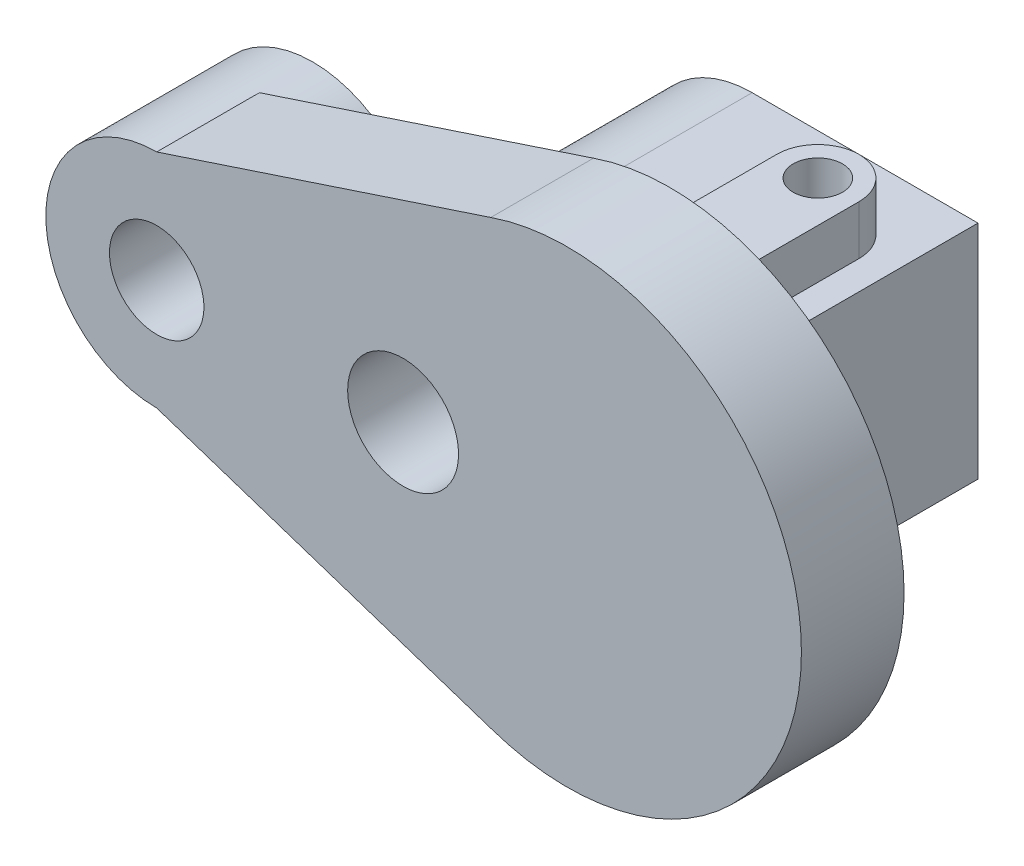
ISO-10303-21;
HEADER;
FILE_DESCRIPTION(('STEP AP214'),'2;1');
FILE_NAME('part.step','',(''),(''),'','','');
FILE_SCHEMA(('AUTOMOTIVE_DESIGN { 1 0 10303 214 1 1 1 1 }'));
ENDSEC;
DATA;
#1=APPLICATION_CONTEXT('core data for automotive mechanical design processes');
#2=APPLICATION_PROTOCOL_DEFINITION('international standard','automotive_design',2000,#1);
#3=PRODUCT_CONTEXT('',#1,'mechanical');
#4=PRODUCT('Part','Part','',(#3));
#5=PRODUCT_RELATED_PRODUCT_CATEGORY('part','',(#4));
#6=PRODUCT_DEFINITION_FORMATION('','',#4);
#7=PRODUCT_DEFINITION_CONTEXT('part definition',#1,'design');
#8=PRODUCT_DEFINITION('design','',#6,#7);
#9=PRODUCT_DEFINITION_SHAPE('','',#8);
#10=(LENGTH_UNIT() NAMED_UNIT(*) SI_UNIT(.MILLI.,.METRE.));
#11=(NAMED_UNIT(*) PLANE_ANGLE_UNIT() SI_UNIT($,.RADIAN.));
#12=(NAMED_UNIT(*) SI_UNIT($,.STERADIAN.) SOLID_ANGLE_UNIT());
#13=UNCERTAINTY_MEASURE_WITH_UNIT(LENGTH_MEASURE(1.E-05),#10,'distance_accuracy_value','');
#14=(GEOMETRIC_REPRESENTATION_CONTEXT(3) GLOBAL_UNCERTAINTY_ASSIGNED_CONTEXT((#13)) GLOBAL_UNIT_ASSIGNED_CONTEXT((#10,
#11,#12)) REPRESENTATION_CONTEXT('',''));
#15=CARTESIAN_POINT('',(0.,0.,0.));
#16=DIRECTION('',(0.,0.,1.));
#17=DIRECTION('',(1.,0.,0.));
#18=AXIS2_PLACEMENT_3D('',#15,#16,#17);
#19=CARTESIAN_POINT('',(115000.,27000.,-66000.));
#20=DIRECTION('',(0.,-1.,0.));
#21=DIRECTION('',(0.,0.,-1.));
#22=AXIS2_PLACEMENT_3D('',#19,#20,#21);
#23=PLANE('',#22);
#24=DIRECTION('',(0.,0.,-1.));
#25=VECTOR('',#24,1.);
#26=CARTESIAN_POINT('',(108000.,27000.,-6000.));
#27=LINE('',#26,#25);
#28=CARTESIAN_POINT('',(108000.,27000.,-11000.));
#29=VERTEX_POINT('',#28);
#30=CARTESIAN_POINT('',(108000.,27000.,-44000.));
#31=VERTEX_POINT('',#30);
#32=EDGE_CURVE('E187',#29,#31,#27,.T.);
#33=ORIENTED_EDGE('',*,*,#32,.F.);
#34=DIRECTION('',(1.,0.,0.));
#35=VECTOR('',#34,1.);
#36=CARTESIAN_POINT('',(-27000.001,27000.,-11000.));
#37=LINE('',#36,#35);
#38=CARTESIAN_POINT('',(115000.,27000.,-11000.));
#39=VERTEX_POINT('',#38);
#40=EDGE_CURVE('E204',#29,#39,#37,.T.);
#41=ORIENTED_EDGE('',*,*,#40,.T.);
#42=DIRECTION('',(0.,0.,1.));
#43=VECTOR('',#42,1.);
#44=CARTESIAN_POINT('',(115000.,27000.,-66000.));
#45=LINE('',#44,#43);
#46=CARTESIAN_POINT('',(115000.,27000.,-66000.));
#47=VERTEX_POINT('',#46);
#48=EDGE_CURVE('E227',#47,#39,#45,.T.);
#49=ORIENTED_EDGE('',*,*,#48,.F.);
#50=DIRECTION('',(1.,0.,0.));
#51=VECTOR('',#50,1.);
#52=CARTESIAN_POINT('',(115000.,27000.,-66000.));
#53=LINE('',#52,#51);
#54=CARTESIAN_POINT('',(60000.,27000.,-66000.));
#55=VERTEX_POINT('',#54);
#56=EDGE_CURVE('E213',#55,#47,#53,.T.);
#57=ORIENTED_EDGE('',*,*,#56,.F.);
#58=DIRECTION('',(0.,0.,1.));
#59=VECTOR('',#58,1.);
#60=CARTESIAN_POINT('',(60000.,27000.,-66000.));
#61=LINE('',#60,#59);
#62=CARTESIAN_POINT('',(60000.,27000.,-11000.));
#63=VERTEX_POINT('',#62);
#64=EDGE_CURVE('E229',#55,#63,#61,.T.);
#65=ORIENTED_EDGE('',*,*,#64,.T.);
#66=CARTESIAN_POINT('',(88000.,27000.,-11000.));
#67=VERTEX_POINT('',#66);
#68=EDGE_CURVE('E201',#63,#67,#37,.T.);
#69=ORIENTED_EDGE('',*,*,#68,.T.);
#70=DIRECTION('',(0.,0.,1.));
#71=VECTOR('',#70,1.);
#72=CARTESIAN_POINT('',(88000.,27000.,-6000.));
#73=LINE('',#72,#71);
#74=CARTESIAN_POINT('',(88000.,27000.,-44000.));
#75=VERTEX_POINT('',#74);
#76=EDGE_CURVE('E563',#75,#67,#73,.T.);
#77=ORIENTED_EDGE('',*,*,#76,.F.);
#78=CARTESIAN_POINT('',(98000.,27000.,-44000.));
#79=DIRECTION('',(0.,1.,0.));
#80=DIRECTION('',(0.,0.,1.));
#81=AXIS2_PLACEMENT_3D('',#78,#79,#80);
#82=CIRCLE('',#81,10000.);
#83=EDGE_CURVE('E557',#31,#75,#82,.T.);
#84=ORIENTED_EDGE('',*,*,#83,.F.);
#85=EDGE_LOOP('',(#33,#41,#49,#57,#65,#69,#77,#84));
#86=FACE_BOUND('',#85,.T.);
#87=ADVANCED_FACE('F41',(#86),#23,.F.);
#88=CARTESIAN_POINT('',(98000.,-27000.,-44000.));
#89=DIRECTION('',(0.,-1.,0.));
#90=DIRECTION('',(0.,0.,-1.));
#91=AXIS2_PLACEMENT_3D('',#88,#89,#90);
#92=PLANE('',#91);
#93=DIRECTION('',(1.,0.,0.));
#94=VECTOR('',#93,1.);
#95=CARTESIAN_POINT('',(98000.,-27000.,-11000.));
#96=LINE('',#95,#94);
#97=CARTESIAN_POINT('',(88000.,-27000.,-11000.));
#98=VERTEX_POINT('',#97);
#99=CARTESIAN_POINT('',(108000.,-27000.,-11000.));
#100=VERTEX_POINT('',#99);
#101=EDGE_CURVE('E11',#98,#100,#96,.T.);
#102=ORIENTED_EDGE('',*,*,#101,.F.);
#103=DIRECTION('',(0.,0.,-1.));
#104=VECTOR('',#103,1.);
#105=CARTESIAN_POINT('',(88000.,-27000.,-6000.));
#106=LINE('',#105,#104);
#107=CARTESIAN_POINT('',(88000.,-27000.,-6000.));
#108=VERTEX_POINT('',#107);
#109=EDGE_CURVE('E252',#108,#98,#106,.T.);
#110=ORIENTED_EDGE('',*,*,#109,.F.);
#111=DIRECTION('',(-1.,0.,0.));
#112=VECTOR('',#111,1.);
#113=CARTESIAN_POINT('',(108000.,-27000.,-6000.));
#114=LINE('',#113,#112);
#115=CARTESIAN_POINT('',(108000.,-27000.,-6000.));
#116=VERTEX_POINT('',#115);
#117=EDGE_CURVE('E247',#116,#108,#114,.T.);
#118=ORIENTED_EDGE('',*,*,#117,.F.);
#119=DIRECTION('',(0.,0.,1.));
#120=VECTOR('',#119,1.);
#121=CARTESIAN_POINT('',(108000.,-27000.,-6000.));
#122=LINE('',#121,#120);
#123=EDGE_CURVE('E231',#100,#116,#122,.T.);
#124=ORIENTED_EDGE('',*,*,#123,.F.);
#125=EDGE_LOOP('',(#102,#110,#118,#124));
#126=FACE_BOUND('',#125,.T.);
#127=ADVANCED_FACE('F354',(#126),#92,.F.);
#128=CARTESIAN_POINT('',(0.,0.,-6000.));
#129=DIRECTION('',(0.,0.,1.));
#130=DIRECTION('',(1.,0.,0.));
#131=AXIS2_PLACEMENT_3D('',#128,#129,#130);
#132=PLANE('',#131);
#133=DIRECTION('',(0.,-1.,0.));
#134=VECTOR('',#133,1.);
#135=CARTESIAN_POINT('',(108000.,39000.,-6000.));
#136=LINE('',#135,#134);
#137=CARTESIAN_POINT('',(108000.,39000.,-6000.));
#138=VERTEX_POINT('',#137);
#139=CARTESIAN_POINT('',(108000.,27000.,-6000.));
#140=VERTEX_POINT('',#139);
#141=EDGE_CURVE('E57',#138,#140,#136,.T.);
#142=ORIENTED_EDGE('',*,*,#141,.F.);
#143=DIRECTION('',(1.,0.,0.));
#144=VECTOR('',#143,1.);
#145=CARTESIAN_POINT('',(108000.,39000.,-6000.));
#146=LINE('',#145,#144);
#147=CARTESIAN_POINT('',(88000.,39000.,-6000.));
#148=VERTEX_POINT('',#147);
#149=EDGE_CURVE('E58',#148,#138,#146,.T.);
#150=ORIENTED_EDGE('',*,*,#149,.F.);
#151=DIRECTION('',(0.,-1.,0.));
#152=VECTOR('',#151,1.);
#153=CARTESIAN_POINT('',(88000.,39000.,-6000.));
#154=LINE('',#153,#152);
#155=CARTESIAN_POINT('',(88000.,27000.,-6000.));
#156=VERTEX_POINT('',#155);
#157=EDGE_CURVE('E195',#148,#156,#154,.T.);
#158=ORIENTED_EDGE('',*,*,#157,.T.);
#159=DIRECTION('',(1.,0.,0.));
#160=VECTOR('',#159,1.);
#161=CARTESIAN_POINT('',(108000.,27000.,-6000.));
#162=LINE('',#161,#160);
#163=EDGE_CURVE('E179',#156,#140,#162,.T.);
#164=ORIENTED_EDGE('',*,*,#163,.T.);
#165=EDGE_LOOP('',(#142,#150,#158,#164));
#166=FACE_BOUND('',#165,.T.);
#167=DIRECTION('',(0.,1.,0.));
#168=VECTOR('',#167,1.);
#169=CARTESIAN_POINT('',(88000.,-39000.,-6000.));
#170=LINE('',#169,#168);
#171=CARTESIAN_POINT('',(88000.,-39000.,-6000.));
#172=VERTEX_POINT('',#171);
#173=EDGE_CURVE('E258',#172,#108,#170,.T.);
#174=ORIENTED_EDGE('',*,*,#173,.F.);
#175=DIRECTION('',(-1.,0.,0.));
#176=VECTOR('',#175,1.);
#177=CARTESIAN_POINT('',(108000.,-39000.,-6000.));
#178=LINE('',#177,#176);
#179=CARTESIAN_POINT('',(108000.,-39000.,-6000.));
#180=VERTEX_POINT('',#179);
#181=EDGE_CURVE('E240',#180,#172,#178,.T.);
#182=ORIENTED_EDGE('',*,*,#181,.F.);
#183=DIRECTION('',(0.,1.,0.));
#184=VECTOR('',#183,1.);
#185=CARTESIAN_POINT('',(108000.,-39000.,-6000.));
#186=LINE('',#185,#184);
#187=EDGE_CURVE('E261',#180,#116,#186,.T.);
#188=ORIENTED_EDGE('',*,*,#187,.T.);
#189=ORIENTED_EDGE('',*,*,#117,.T.);
#190=EDGE_LOOP('',(#174,#182,#188,#189));
#191=FACE_BOUND('',#190,.T.);
#192=CARTESIAN_POINT('',(0.,0.,-6000.));
#193=DIRECTION('',(0.,0.,-1.));
#194=DIRECTION('',(1.,0.,0.));
#195=AXIS2_PLACEMENT_3D('',#192,#193,#194);
#196=CIRCLE('',#195,27000.);
#197=CARTESIAN_POINT('',(0.,27000.,-6000.));
#198=VERTEX_POINT('',#197);
#199=CARTESIAN_POINT('',(0.,-27000.,-6000.));
#200=VERTEX_POINT('',#199);
#201=EDGE_CURVE('E267',#198,#200,#196,.T.);
#202=ORIENTED_EDGE('',*,*,#201,.F.);
#203=DIRECTION('',(-0.949568733780847,-0.313558957495777,0.));
#204=VECTOR('',#203,1.);
#205=CARTESIAN_POINT('',(0.,27000.,-6000.));
#206=LINE('',#205,#204);
#207=CARTESIAN_POINT('',(81360.2667835362,53866.1335684961,-6000.));
#208=VERTEX_POINT('',#207);
#209=EDGE_CURVE('E289',#208,#198,#206,.T.);
#210=ORIENTED_EDGE('',*,*,#209,.F.);
#211=CARTESIAN_POINT('',(100000.,0.,-6000.));
#212=DIRECTION('',(0.,0.,1.));
#213=DIRECTION('',(1.,0.,0.));
#214=AXIS2_PLACEMENT_3D('',#211,#212,#213);
#215=CIRCLE('',#214,57000.);
#216=CARTESIAN_POINT('',(81360.2667835362,-53866.1335684961,-6000.));
#217=VERTEX_POINT('',#216);
#218=EDGE_CURVE('E284',#217,#208,#215,.T.);
#219=ORIENTED_EDGE('',*,*,#218,.F.);
#220=DIRECTION('',(0.949568733780847,-0.313558957495777,0.));
#221=VECTOR('',#220,1.);
#222=CARTESIAN_POINT('',(0.,-27000.,-6000.));
#223=LINE('',#222,#221);
#224=EDGE_CURVE('E285',#200,#217,#223,.T.);
#225=ORIENTED_EDGE('',*,*,#224,.F.);
#226=EDGE_LOOP('',(#202,#210,#219,#225));
#227=FACE_BOUND('',#226,.T.);
#228=CARTESIAN_POINT('',(60000.,-1.4210854715202E-11,-6000.));
#229=DIRECTION('',(0.,0.,1.));
#230=DIRECTION('',(1.,0.,0.));
#231=AXIS2_PLACEMENT_3D('',#228,#229,#230);
#232=CIRCLE('',#231,13500.);
#233=CARTESIAN_POINT('',(73500.,-1.4210854715202E-11,-6000.));
#234=VERTEX_POINT('',#233);
#235=EDGE_CURVE('E47',#234,#234,#232,.T.);
#236=ORIENTED_EDGE('',*,*,#235,.T.);
#237=EDGE_LOOP('',(#236));
#238=FACE_BOUND('',#237,.T.);
#239=ADVANCED_FACE('F312',(#166,#191,#227,#238),#132,.F.);
#240=CARTESIAN_POINT('',(0.,0.,19000.));
#241=DIRECTION('',(0.,0.,-1.));
#242=DIRECTION('',(-1.,0.,0.));
#243=AXIS2_PLACEMENT_3D('',#240,#241,#242);
#244=CYLINDRICAL_SURFACE('',#243,27000.);
#245=CARTESIAN_POINT('',(0.,0.,19000.));
#246=DIRECTION('',(0.,0.,1.));
#247=DIRECTION('',(1.,0.,0.));
#248=AXIS2_PLACEMENT_3D('',#245,#246,#247);
#249=CIRCLE('',#248,27000.);
#250=CARTESIAN_POINT('',(0.,27000.,19000.));
#251=VERTEX_POINT('',#250);
#252=CARTESIAN_POINT('',(0.,-27000.,19000.));
#253=VERTEX_POINT('',#252);
#254=EDGE_CURVE('E275',#251,#253,#249,.T.);
#255=ORIENTED_EDGE('',*,*,#254,.F.);
#256=DIRECTION('',(0.,0.,1.));
#257=VECTOR('',#256,1.);
#258=CARTESIAN_POINT('',(0.,27000.,-6000.));
#259=LINE('',#258,#257);
#260=EDGE_CURVE('E287',#198,#251,#259,.T.);
#261=ORIENTED_EDGE('',*,*,#260,.F.);
#262=ORIENTED_EDGE('',*,*,#201,.T.);
#263=DIRECTION('',(0.,0.,1.));
#264=VECTOR('',#263,1.);
#265=CARTESIAN_POINT('',(0.,-27000.,-6000.));
#266=LINE('',#265,#264);
#267=EDGE_CURVE('E272',#200,#253,#266,.T.);
#268=ORIENTED_EDGE('',*,*,#267,.T.);
#269=EDGE_LOOP('',(#255,#261,#262,#268));
#270=FACE_BOUND('',#269,.T.);
#271=CARTESIAN_POINT('',(0.,0.,-19000.));
#272=DIRECTION('',(0.,0.,1.));
#273=DIRECTION('',(1.,0.,0.));
#274=AXIS2_PLACEMENT_3D('',#271,#272,#273);
#275=CIRCLE('',#274,27000.);
#276=CARTESIAN_POINT('',(27000.,0.,-19000.));
#277=VERTEX_POINT('',#276);
#278=EDGE_CURVE('E270',#277,#277,#275,.T.);
#279=ORIENTED_EDGE('',*,*,#278,.T.);
#280=EDGE_LOOP('',(#279));
#281=FACE_BOUND('',#280,.T.);
#282=ADVANCED_FACE('F323',(#270,#281),#244,.T.);
#283=CARTESIAN_POINT('',(0.,0.,19000.));
#284=DIRECTION('',(0.,0.,1.));
#285=DIRECTION('',(1.,0.,0.));
#286=AXIS2_PLACEMENT_3D('',#283,#284,#285);
#287=PLANE('',#286);
#288=CARTESIAN_POINT('',(0.,0.,19000.));
#289=DIRECTION('',(0.,0.,-1.));
#290=DIRECTION('',(-1.,0.,0.));
#291=AXIS2_PLACEMENT_3D('',#288,#289,#290);
#292=CIRCLE('',#291,11500.);
#293=CARTESIAN_POINT('',(-11500.,0.,19000.));
#294=VERTEX_POINT('',#293);
#295=EDGE_CURVE('E266',#294,#294,#292,.T.);
#296=ORIENTED_EDGE('',*,*,#295,.T.);
#297=EDGE_LOOP('',(#296));
#298=FACE_BOUND('',#297,.T.);
#299=CARTESIAN_POINT('',(60000.,-1.4210854715202E-11,19000.));
#300=DIRECTION('',(0.,0.,-1.));
#301=DIRECTION('',(-1.,0.,0.));
#302=AXIS2_PLACEMENT_3D('',#299,#300,#301);
#303=CIRCLE('',#302,13500.);
#304=CARTESIAN_POINT('',(46500.,-1.4210854715202E-11,19000.));
#305=VERTEX_POINT('',#304);
#306=EDGE_CURVE('E277',#305,#305,#303,.T.);
#307=ORIENTED_EDGE('',*,*,#306,.T.);
#308=EDGE_LOOP('',(#307));
#309=FACE_BOUND('',#308,.T.);
#310=ORIENTED_EDGE('',*,*,#254,.T.);
#311=DIRECTION('',(0.949568733780847,-0.313558957495777,0.));
#312=VECTOR('',#311,1.);
#313=CARTESIAN_POINT('',(0.,-27000.,19000.));
#314=LINE('',#313,#312);
#315=CARTESIAN_POINT('',(81360.2667835362,-53866.1335684961,19000.));
#316=VERTEX_POINT('',#315);
#317=EDGE_CURVE('E273',#253,#316,#314,.T.);
#318=ORIENTED_EDGE('',*,*,#317,.T.);
#319=CARTESIAN_POINT('',(100000.,0.,19000.));
#320=DIRECTION('',(0.,0.,1.));
#321=DIRECTION('',(1.,0.,0.));
#322=AXIS2_PLACEMENT_3D('',#319,#320,#321);
#323=CIRCLE('',#322,57000.);
#324=CARTESIAN_POINT('',(81360.2667835362,53866.1335684961,19000.));
#325=VERTEX_POINT('',#324);
#326=EDGE_CURVE('E292',#316,#325,#323,.T.);
#327=ORIENTED_EDGE('',*,*,#326,.T.);
#328=DIRECTION('',(-0.949568733780847,-0.313558957495777,0.));
#329=VECTOR('',#328,1.);
#330=CARTESIAN_POINT('',(0.,27000.,19000.));
#331=LINE('',#330,#329);
#332=EDGE_CURVE('E286',#325,#251,#331,.T.);
#333=ORIENTED_EDGE('',*,*,#332,.T.);
#334=EDGE_LOOP('',(#310,#318,#327,#333));
#335=FACE_BOUND('',#334,.T.);
#336=ADVANCED_FACE('F322',(#298,#309,#335),#287,.T.);
#337=CARTESIAN_POINT('',(0.,0.,-19000.));
#338=DIRECTION('',(0.,0.,1.));
#339=DIRECTION('',(1.,0.,0.));
#340=AXIS2_PLACEMENT_3D('',#337,#338,#339);
#341=PLANE('',#340);
#342=CARTESIAN_POINT('',(0.,0.,-19000.));
#343=DIRECTION('',(0.,0.,-1.));
#344=DIRECTION('',(-1.,0.,0.));
#345=AXIS2_PLACEMENT_3D('',#342,#343,#344);
#346=CIRCLE('',#345,11500.);
#347=CARTESIAN_POINT('',(-11500.,0.,-19000.));
#348=VERTEX_POINT('',#347);
#349=EDGE_CURVE('E283',#348,#348,#346,.T.);
#350=ORIENTED_EDGE('',*,*,#349,.F.);
#351=EDGE_LOOP('',(#350));
#352=FACE_BOUND('',#351,.T.);
#353=ORIENTED_EDGE('',*,*,#278,.F.);
#354=EDGE_LOOP('',(#353));
#355=FACE_BOUND('',#354,.T.);
#356=ADVANCED_FACE('F321',(#352,#355),#341,.F.);
#357=CARTESIAN_POINT('',(0.,27000.,-6000.));
#358=DIRECTION('',(-0.313558957495777,0.949568733780847,0.));
#359=DIRECTION('',(-0.949568733780847,-0.313558957495777,0.));
#360=AXIS2_PLACEMENT_3D('',#357,#358,#359);
#361=PLANE('',#360);
#362=ORIENTED_EDGE('',*,*,#332,.F.);
#363=DIRECTION('',(0.,0.,1.));
#364=VECTOR('',#363,1.);
#365=CARTESIAN_POINT('',(81360.2667835362,53866.1335684961,-6000.));
#366=LINE('',#365,#364);
#367=EDGE_CURVE('E281',#208,#325,#366,.T.);
#368=ORIENTED_EDGE('',*,*,#367,.F.);
#369=ORIENTED_EDGE('',*,*,#209,.T.);
#370=ORIENTED_EDGE('',*,*,#260,.T.);
#371=EDGE_LOOP('',(#362,#368,#369,#370));
#372=FACE_BOUND('',#371,.T.);
#373=ADVANCED_FACE('F345',(#372),#361,.T.);
#374=CARTESIAN_POINT('',(100000.,0.,-6000.));
#375=DIRECTION('',(0.,0.,1.));
#376=DIRECTION('',(1.,0.,0.));
#377=AXIS2_PLACEMENT_3D('',#374,#375,#376);
#378=CYLINDRICAL_SURFACE('',#377,57000.);
#379=ORIENTED_EDGE('',*,*,#326,.F.);
#380=DIRECTION('',(0.,0.,1.));
#381=VECTOR('',#380,1.);
#382=CARTESIAN_POINT('',(81360.2667835362,-53866.1335684961,-6000.));
#383=LINE('',#382,#381);
#384=EDGE_CURVE('E276',#217,#316,#383,.T.);
#385=ORIENTED_EDGE('',*,*,#384,.F.);
#386=ORIENTED_EDGE('',*,*,#218,.T.);
#387=ORIENTED_EDGE('',*,*,#367,.T.);
#388=EDGE_LOOP('',(#379,#385,#386,#387));
#389=FACE_BOUND('',#388,.T.);
#390=ADVANCED_FACE('F338',(#389),#378,.T.);
#391=CARTESIAN_POINT('',(0.,-27000.,-6000.));
#392=DIRECTION('',(-0.313558957495777,-0.949568733780847,0.));
#393=DIRECTION('',(0.949568733780847,-0.313558957495777,0.));
#394=AXIS2_PLACEMENT_3D('',#391,#392,#393);
#395=PLANE('',#394);
#396=ORIENTED_EDGE('',*,*,#317,.F.);
#397=ORIENTED_EDGE('',*,*,#267,.F.);
#398=ORIENTED_EDGE('',*,*,#224,.T.);
#399=ORIENTED_EDGE('',*,*,#384,.T.);
#400=EDGE_LOOP('',(#396,#397,#398,#399));
#401=FACE_BOUND('',#400,.T.);
#402=ADVANCED_FACE('F319',(#401),#395,.T.);
#403=CARTESIAN_POINT('',(60000.,-1.4210854715202E-11,19000.));
#404=DIRECTION('',(0.,0.,-1.));
#405=DIRECTION('',(-1.,0.,0.));
#406=AXIS2_PLACEMENT_3D('',#403,#404,#405);
#407=CYLINDRICAL_SURFACE('',#406,13500.);
#408=ORIENTED_EDGE('',*,*,#235,.F.);
#409=EDGE_LOOP('',(#408));
#410=FACE_BOUND('',#409,.T.);
#411=ORIENTED_EDGE('',*,*,#306,.F.);
#412=EDGE_LOOP('',(#411));
#413=FACE_BOUND('',#412,.T.);
#414=ADVANCED_FACE('F43',(#410,#413),#407,.F.);
#415=CARTESIAN_POINT('',(0.,0.,19000.));
#416=DIRECTION('',(0.,0.,-1.));
#417=DIRECTION('',(-1.,0.,0.));
#418=AXIS2_PLACEMENT_3D('',#415,#416,#417);
#419=CYLINDRICAL_SURFACE('',#418,11500.);
#420=ORIENTED_EDGE('',*,*,#295,.F.);
#421=EDGE_LOOP('',(#420));
#422=FACE_BOUND('',#421,.T.);
#423=ORIENTED_EDGE('',*,*,#349,.T.);
#424=EDGE_LOOP('',(#423));
#425=FACE_BOUND('',#424,.T.);
#426=ADVANCED_FACE('F320',(#422,#425),#419,.F.);
#427=CARTESIAN_POINT('',(108000.,-39000.,-6000.));
#428=DIRECTION('',(-1.,0.,0.));
#429=DIRECTION('',(0.,0.,1.));
#430=AXIS2_PLACEMENT_3D('',#427,#428,#429);
#431=PLANE('',#430);
#432=CARTESIAN_POINT('',(108000.,-27000.,-44000.));
#433=VERTEX_POINT('',#432);
#434=EDGE_CURVE('E246',#433,#100,#122,.T.);
#435=ORIENTED_EDGE('',*,*,#434,.T.);
#436=ORIENTED_EDGE('',*,*,#123,.T.);
#437=ORIENTED_EDGE('',*,*,#187,.F.);
#438=DIRECTION('',(0.,0.,1.));
#439=VECTOR('',#438,1.);
#440=CARTESIAN_POINT('',(108000.,-39000.,-6000.));
#441=LINE('',#440,#439);
#442=CARTESIAN_POINT('',(108000.,-39000.,-44000.));
#443=VERTEX_POINT('',#442);
#444=EDGE_CURVE('E234',#443,#180,#441,.T.);
#445=ORIENTED_EDGE('',*,*,#444,.F.);
#446=DIRECTION('',(0.,1.,0.));
#447=VECTOR('',#446,1.);
#448=CARTESIAN_POINT('',(108000.,-39000.,-44000.));
#449=LINE('',#448,#447);
#450=EDGE_CURVE('E244',#443,#433,#449,.T.);
#451=ORIENTED_EDGE('',*,*,#450,.T.);
#452=EDGE_LOOP('',(#435,#436,#437,#445,#451));
#453=FACE_BOUND('',#452,.T.);
#454=ADVANCED_FACE('F383',(#453),#431,.F.);
#455=CARTESIAN_POINT('',(88000.,-39000.,-6000.));
#456=DIRECTION('',(1.,0.,0.));
#457=DIRECTION('',(0.,0.,-1.));
#458=AXIS2_PLACEMENT_3D('',#455,#456,#457);
#459=PLANE('',#458);
#460=ORIENTED_EDGE('',*,*,#109,.T.);
#461=CARTESIAN_POINT('',(88000.,-27000.,-44000.));
#462=VERTEX_POINT('',#461);
#463=EDGE_CURVE('E249',#98,#462,#106,.T.);
#464=ORIENTED_EDGE('',*,*,#463,.T.);
#465=DIRECTION('',(0.,1.,0.));
#466=VECTOR('',#465,1.);
#467=CARTESIAN_POINT('',(88000.,-39000.,-44000.));
#468=LINE('',#467,#466);
#469=CARTESIAN_POINT('',(88000.,-39000.,-44000.));
#470=VERTEX_POINT('',#469);
#471=EDGE_CURVE('E260',#470,#462,#468,.T.);
#472=ORIENTED_EDGE('',*,*,#471,.F.);
#473=DIRECTION('',(0.,0.,-1.));
#474=VECTOR('',#473,1.);
#475=CARTESIAN_POINT('',(88000.,-39000.,-6000.));
#476=LINE('',#475,#474);
#477=EDGE_CURVE('E241',#172,#470,#476,.T.);
#478=ORIENTED_EDGE('',*,*,#477,.F.);
#479=ORIENTED_EDGE('',*,*,#173,.T.);
#480=EDGE_LOOP('',(#460,#464,#472,#478,#479));
#481=FACE_BOUND('',#480,.T.);
#482=ADVANCED_FACE('F382',(#481),#459,.F.);
#483=CARTESIAN_POINT('',(98000.,-39000.,-44000.));
#484=DIRECTION('',(0.,1.,0.));
#485=DIRECTION('',(0.,0.,1.));
#486=AXIS2_PLACEMENT_3D('',#483,#484,#485);
#487=CYLINDRICAL_SURFACE('',#486,10000.);
#488=CARTESIAN_POINT('',(98000.,-27000.,-44000.));
#489=DIRECTION('',(0.,-1.,0.));
#490=DIRECTION('',(0.,0.,-1.));
#491=AXIS2_PLACEMENT_3D('',#488,#489,#490);
#492=CIRCLE('',#491,10000.);
#493=EDGE_CURVE('E238',#462,#433,#492,.T.);
#494=ORIENTED_EDGE('',*,*,#493,.T.);
#495=ORIENTED_EDGE('',*,*,#450,.F.);
#496=CARTESIAN_POINT('',(98000.,-39000.,-44000.));
#497=DIRECTION('',(0.,-1.,0.));
#498=DIRECTION('',(0.,0.,-1.));
#499=AXIS2_PLACEMENT_3D('',#496,#497,#498);
#500=CIRCLE('',#499,10000.);
#501=EDGE_CURVE('E243',#470,#443,#500,.T.);
#502=ORIENTED_EDGE('',*,*,#501,.F.);
#503=ORIENTED_EDGE('',*,*,#471,.T.);
#504=EDGE_LOOP('',(#494,#495,#502,#503));
#505=FACE_BOUND('',#504,.T.);
#506=ADVANCED_FACE('F376',(#505),#487,.T.);
#507=CARTESIAN_POINT('',(98000.,-39000.,-44000.));
#508=DIRECTION('',(0.,-1.,0.));
#509=DIRECTION('',(0.,0.,-1.));
#510=AXIS2_PLACEMENT_3D('',#507,#508,#509);
#511=PLANE('',#510);
#512=CARTESIAN_POINT('',(98000.,-39000.,-44000.));
#513=DIRECTION('',(0.,-1.,0.));
#514=DIRECTION('',(0.,0.,-1.));
#515=AXIS2_PLACEMENT_3D('',#512,#513,#514);
#516=CIRCLE('',#515,5999.99999999999);
#517=CARTESIAN_POINT('',(98000.,-39000.,-50000.));
#518=VERTEX_POINT('',#517);
#519=EDGE_CURVE('E549',#518,#518,#516,.T.);
#520=ORIENTED_EDGE('',*,*,#519,.F.);
#521=EDGE_LOOP('',(#520));
#522=FACE_BOUND('',#521,.T.);
#523=ORIENTED_EDGE('',*,*,#444,.T.);
#524=ORIENTED_EDGE('',*,*,#181,.T.);
#525=ORIENTED_EDGE('',*,*,#477,.T.);
#526=ORIENTED_EDGE('',*,*,#501,.T.);
#527=EDGE_LOOP('',(#523,#524,#525,#526));
#528=FACE_BOUND('',#527,.T.);
#529=ADVANCED_FACE('F373',(#522,#528),#511,.T.);
#530=CARTESIAN_POINT('',(115000.,-27000.,-66000.));
#531=DIRECTION('',(0.,1.,0.));
#532=DIRECTION('',(0.,0.,1.));
#533=AXIS2_PLACEMENT_3D('',#530,#531,#532);
#534=PLANE('',#533);
#535=DIRECTION('',(1.,0.,0.));
#536=VECTOR('',#535,1.);
#537=CARTESIAN_POINT('',(-27000.001,-27000.,-11000.));
#538=LINE('',#537,#536);
#539=CARTESIAN_POINT('',(115000.,-27000.,-11000.));
#540=VERTEX_POINT('',#539);
#541=EDGE_CURVE('E188',#100,#540,#538,.T.);
#542=ORIENTED_EDGE('',*,*,#541,.F.);
#543=ORIENTED_EDGE('',*,*,#434,.F.);
#544=ORIENTED_EDGE('',*,*,#493,.F.);
#545=ORIENTED_EDGE('',*,*,#463,.F.);
#546=CARTESIAN_POINT('',(60000.,-27000.,-11000.));
#547=VERTEX_POINT('',#546);
#548=EDGE_CURVE('E202',#547,#98,#538,.T.);
#549=ORIENTED_EDGE('',*,*,#548,.F.);
#550=DIRECTION('',(0.,0.,1.));
#551=VECTOR('',#550,1.);
#552=CARTESIAN_POINT('',(60000.,-27000.,-66000.));
#553=LINE('',#552,#551);
#554=CARTESIAN_POINT('',(60000.,-27000.,-66000.));
#555=VERTEX_POINT('',#554);
#556=EDGE_CURVE('E222',#555,#547,#553,.T.);
#557=ORIENTED_EDGE('',*,*,#556,.F.);
#558=DIRECTION('',(-1.,0.,0.));
#559=VECTOR('',#558,1.);
#560=CARTESIAN_POINT('',(115000.,-27000.,-66000.));
#561=LINE('',#560,#559);
#562=CARTESIAN_POINT('',(115000.,-27000.,-66000.));
#563=VERTEX_POINT('',#562);
#564=EDGE_CURVE('E217',#563,#555,#561,.T.);
#565=ORIENTED_EDGE('',*,*,#564,.F.);
#566=DIRECTION('',(0.,0.,1.));
#567=VECTOR('',#566,1.);
#568=CARTESIAN_POINT('',(115000.,-27000.,-66000.));
#569=LINE('',#568,#567);
#570=EDGE_CURVE('E224',#563,#540,#569,.T.);
#571=ORIENTED_EDGE('',*,*,#570,.T.);
#572=EDGE_LOOP('',(#542,#543,#544,#545,#549,#557,#565,#571));
#573=FACE_BOUND('',#572,.T.);
#574=ADVANCED_FACE('F374',(#573),#534,.F.);
#575=CARTESIAN_POINT('',(115000.,27000.,-66000.));
#576=DIRECTION('',(-1.,0.,0.));
#577=DIRECTION('',(0.,0.,1.));
#578=AXIS2_PLACEMENT_3D('',#575,#576,#577);
#579=PLANE('',#578);
#580=ORIENTED_EDGE('',*,*,#48,.T.);
#581=DIRECTION('',(0.,1.,0.));
#582=VECTOR('',#581,1.);
#583=CARTESIAN_POINT('',(115000.,27000.,-11000.));
#584=LINE('',#583,#582);
#585=EDGE_CURVE('E190',#540,#39,#584,.T.);
#586=ORIENTED_EDGE('',*,*,#585,.F.);
#587=ORIENTED_EDGE('',*,*,#570,.F.);
#588=DIRECTION('',(0.,-1.,0.));
#589=VECTOR('',#588,1.);
#590=CARTESIAN_POINT('',(115000.,27000.,-66000.));
#591=LINE('',#590,#589);
#592=EDGE_CURVE('E220',#47,#563,#591,.T.);
#593=ORIENTED_EDGE('',*,*,#592,.F.);
#594=EDGE_LOOP('',(#580,#586,#587,#593));
#595=FACE_BOUND('',#594,.T.);
#596=ADVANCED_FACE('F366',(#595),#579,.F.);
#597=CARTESIAN_POINT('',(60000.,-1.4210854715202E-11,-66000.));
#598=DIRECTION('',(0.,0.,1.));
#599=DIRECTION('',(1.,0.,0.));
#600=AXIS2_PLACEMENT_3D('',#597,#598,#599);
#601=CYLINDRICAL_SURFACE('',#600,27000.);
#602=ORIENTED_EDGE('',*,*,#556,.T.);
#603=CARTESIAN_POINT('',(60000.,-1.4210854715202E-11,-11000.));
#604=DIRECTION('',(0.,0.,-1.));
#605=DIRECTION('',(0.,1.,0.));
#606=AXIS2_PLACEMENT_3D('',#603,#604,#605);
#607=CIRCLE('',#606,27000.);
#608=EDGE_CURVE('E199',#63,#547,#607,.F.);
#609=ORIENTED_EDGE('',*,*,#608,.F.);
#610=ORIENTED_EDGE('',*,*,#64,.F.);
#611=CARTESIAN_POINT('',(60000.,-1.4210854715202E-11,-66000.));
#612=DIRECTION('',(0.,0.,-1.));
#613=DIRECTION('',(-1.,0.,0.));
#614=AXIS2_PLACEMENT_3D('',#611,#612,#613);
#615=CIRCLE('',#614,27000.);
#616=EDGE_CURVE('E215',#555,#55,#615,.T.);
#617=ORIENTED_EDGE('',*,*,#616,.F.);
#618=EDGE_LOOP('',(#602,#609,#610,#617));
#619=FACE_BOUND('',#618,.T.);
#620=ADVANCED_FACE('F368',(#619),#601,.T.);
#621=CARTESIAN_POINT('',(60000.,-1.4210854715202E-11,-66000.));
#622=DIRECTION('',(0.,0.,-1.));
#623=DIRECTION('',(-1.,0.,0.));
#624=AXIS2_PLACEMENT_3D('',#621,#622,#623);
#625=PLANE('',#624);
#626=CARTESIAN_POINT('',(60000.,-1.4210854715202E-11,-66000.));
#627=DIRECTION('',(0.,0.,-1.));
#628=DIRECTION('',(-1.,0.,0.));
#629=AXIS2_PLACEMENT_3D('',#626,#627,#628);
#630=CIRCLE('',#629,13500.);
#631=CARTESIAN_POINT('',(46500.,-1.4210854715202E-11,-66000.));
#632=VERTEX_POINT('',#631);
#633=EDGE_CURVE('E197',#632,#632,#630,.T.);
#634=ORIENTED_EDGE('',*,*,#633,.F.);
#635=EDGE_LOOP('',(#634));
#636=FACE_BOUND('',#635,.T.);
#637=ORIENTED_EDGE('',*,*,#616,.T.);
#638=ORIENTED_EDGE('',*,*,#56,.T.);
#639=ORIENTED_EDGE('',*,*,#592,.T.);
#640=ORIENTED_EDGE('',*,*,#564,.T.);
#641=EDGE_LOOP('',(#637,#638,#639,#640));
#642=FACE_BOUND('',#641,.T.);
#643=ADVANCED_FACE('F371',(#636,#642),#625,.T.);
#644=CARTESIAN_POINT('',(60000.,-1.4210854715202E-11,19000.));
#645=DIRECTION('',(0.,0.,-1.));
#646=DIRECTION('',(-1.,0.,0.));
#647=AXIS2_PLACEMENT_3D('',#644,#645,#646);
#648=CYLINDRICAL_SURFACE('',#647,13500.);
#649=CARTESIAN_POINT('',(60000.,-1.4210854715202E-11,-11000.));
#650=DIRECTION('',(0.,0.,-1.));
#651=DIRECTION('',(0.,1.,0.));
#652=AXIS2_PLACEMENT_3D('',#649,#650,#651);
#653=CIRCLE('',#652,13500.);
#654=CARTESIAN_POINT('',(60000.,13500.,-11000.));
#655=VERTEX_POINT('',#654);
#656=EDGE_CURVE('E198',#655,#655,#653,.T.);
#657=ORIENTED_EDGE('',*,*,#656,.F.);
#658=EDGE_LOOP('',(#657));
#659=FACE_BOUND('',#658,.T.);
#660=ORIENTED_EDGE('',*,*,#633,.T.);
#661=EDGE_LOOP('',(#660));
#662=FACE_BOUND('',#661,.T.);
#663=ADVANCED_FACE('F451',(#659,#662),#648,.F.);
#664=CARTESIAN_POINT('',(-27000.001,27000.,-11000.));
#665=DIRECTION('',(0.,0.,-1.));
#666=DIRECTION('',(0.,1.,0.));
#667=AXIS2_PLACEMENT_3D('',#664,#665,#666);
#668=PLANE('',#667);
#669=ORIENTED_EDGE('',*,*,#608,.T.);
#670=ORIENTED_EDGE('',*,*,#548,.T.);
#671=ORIENTED_EDGE('',*,*,#101,.T.);
#672=ORIENTED_EDGE('',*,*,#541,.T.);
#673=ORIENTED_EDGE('',*,*,#585,.T.);
#674=ORIENTED_EDGE('',*,*,#40,.F.);
#675=EDGE_CURVE('E210',#67,#29,#37,.T.);
#676=ORIENTED_EDGE('',*,*,#675,.F.);
#677=ORIENTED_EDGE('',*,*,#68,.F.);
#678=EDGE_LOOP('',(#669,#670,#671,#672,#673,#674,#676,#677));
#679=FACE_BOUND('',#678,.T.);
#680=ORIENTED_EDGE('',*,*,#656,.T.);
#681=EDGE_LOOP('',(#680));
#682=FACE_BOUND('',#681,.T.);
#683=ADVANCED_FACE('F465',(#679,#682),#668,.F.);
#684=CARTESIAN_POINT('',(98000.,27000.,-44000.));
#685=DIRECTION('',(0.,1.,0.));
#686=DIRECTION('',(0.,0.,1.));
#687=AXIS2_PLACEMENT_3D('',#684,#685,#686);
#688=PLANE('',#687);
#689=EDGE_CURVE('E565',#67,#156,#73,.T.);
#690=ORIENTED_EDGE('',*,*,#689,.F.);
#691=ORIENTED_EDGE('',*,*,#675,.T.);
#692=EDGE_CURVE('E556',#140,#29,#27,.T.);
#693=ORIENTED_EDGE('',*,*,#692,.F.);
#694=ORIENTED_EDGE('',*,*,#163,.F.);
#695=EDGE_LOOP('',(#690,#691,#693,#694));
#696=FACE_BOUND('',#695,.T.);
#697=ADVANCED_FACE('F471',(#696),#688,.F.);
#698=CARTESIAN_POINT('',(108000.,39000.,-6000.));
#699=DIRECTION('',(-1.,0.,0.));
#700=DIRECTION('',(0.,0.,1.));
#701=AXIS2_PLACEMENT_3D('',#698,#699,#700);
#702=PLANE('',#701);
#703=ORIENTED_EDGE('',*,*,#692,.T.);
#704=ORIENTED_EDGE('',*,*,#32,.T.);
#705=DIRECTION('',(0.,-1.,0.));
#706=VECTOR('',#705,1.);
#707=CARTESIAN_POINT('',(108000.,39000.,-44000.));
#708=LINE('',#707,#706);
#709=CARTESIAN_POINT('',(108000.,39000.,-44000.));
#710=VERTEX_POINT('',#709);
#711=EDGE_CURVE('E169',#710,#31,#708,.T.);
#712=ORIENTED_EDGE('',*,*,#711,.F.);
#713=DIRECTION('',(0.,0.,-1.));
#714=VECTOR('',#713,1.);
#715=CARTESIAN_POINT('',(108000.,39000.,-6000.));
#716=LINE('',#715,#714);
#717=EDGE_CURVE('E174',#138,#710,#716,.T.);
#718=ORIENTED_EDGE('',*,*,#717,.F.);
#719=ORIENTED_EDGE('',*,*,#141,.T.);
#720=EDGE_LOOP('',(#703,#704,#712,#718,#719));
#721=FACE_BOUND('',#720,.T.);
#722=ADVANCED_FACE('F183',(#721),#702,.F.);
#723=CARTESIAN_POINT('',(98000.,39000.,-44000.));
#724=DIRECTION('',(0.,-1.,0.));
#725=DIRECTION('',(0.,0.,-1.));
#726=AXIS2_PLACEMENT_3D('',#723,#724,#725);
#727=CYLINDRICAL_SURFACE('',#726,10000.);
#728=ORIENTED_EDGE('',*,*,#83,.T.);
#729=DIRECTION('',(0.,-1.,0.));
#730=VECTOR('',#729,1.);
#731=CARTESIAN_POINT('',(88000.,39000.,-44000.));
#732=LINE('',#731,#730);
#733=CARTESIAN_POINT('',(88000.,39000.,-44000.));
#734=VERTEX_POINT('',#733);
#735=EDGE_CURVE('E171',#734,#75,#732,.T.);
#736=ORIENTED_EDGE('',*,*,#735,.F.);
#737=CARTESIAN_POINT('',(98000.,39000.,-44000.));
#738=DIRECTION('',(0.,1.,0.));
#739=DIRECTION('',(0.,0.,1.));
#740=AXIS2_PLACEMENT_3D('',#737,#738,#739);
#741=CIRCLE('',#740,10000.);
#742=EDGE_CURVE('E165',#710,#734,#741,.T.);
#743=ORIENTED_EDGE('',*,*,#742,.F.);
#744=ORIENTED_EDGE('',*,*,#711,.T.);
#745=EDGE_LOOP('',(#728,#736,#743,#744));
#746=FACE_BOUND('',#745,.T.);
#747=ADVANCED_FACE('F170',(#746),#727,.T.);
#748=CARTESIAN_POINT('',(88000.,39000.,-6000.));
#749=DIRECTION('',(1.,0.,0.));
#750=DIRECTION('',(0.,0.,-1.));
#751=AXIS2_PLACEMENT_3D('',#748,#749,#750);
#752=PLANE('',#751);
#753=ORIENTED_EDGE('',*,*,#76,.T.);
#754=ORIENTED_EDGE('',*,*,#689,.T.);
#755=ORIENTED_EDGE('',*,*,#157,.F.);
#756=DIRECTION('',(0.,0.,1.));
#757=VECTOR('',#756,1.);
#758=CARTESIAN_POINT('',(88000.,39000.,-6000.));
#759=LINE('',#758,#757);
#760=EDGE_CURVE('E172',#734,#148,#759,.T.);
#761=ORIENTED_EDGE('',*,*,#760,.F.);
#762=ORIENTED_EDGE('',*,*,#735,.T.);
#763=EDGE_LOOP('',(#753,#754,#755,#761,#762));
#764=FACE_BOUND('',#763,.T.);
#765=ADVANCED_FACE('F512',(#764),#752,.F.);
#766=CARTESIAN_POINT('',(98000.,39000.,-44000.));
#767=DIRECTION('',(0.,1.,0.));
#768=DIRECTION('',(0.,0.,1.));
#769=AXIS2_PLACEMENT_3D('',#766,#767,#768);
#770=PLANE('',#769);
#771=CARTESIAN_POINT('',(98000.,39000.,-44000.));
#772=DIRECTION('',(0.,1.,0.));
#773=DIRECTION('',(0.,0.,1.));
#774=AXIS2_PLACEMENT_3D('',#771,#772,#773);
#775=CIRCLE('',#774,5999.99999999999);
#776=CARTESIAN_POINT('',(98000.,39000.,-38000.));
#777=VERTEX_POINT('',#776);
#778=EDGE_CURVE('E552',#777,#777,#775,.T.);
#779=ORIENTED_EDGE('',*,*,#778,.F.);
#780=EDGE_LOOP('',(#779));
#781=FACE_BOUND('',#780,.T.);
#782=ORIENTED_EDGE('',*,*,#717,.T.);
#783=ORIENTED_EDGE('',*,*,#742,.T.);
#784=ORIENTED_EDGE('',*,*,#760,.T.);
#785=ORIENTED_EDGE('',*,*,#149,.T.);
#786=EDGE_LOOP('',(#782,#783,#784,#785));
#787=FACE_BOUND('',#786,.T.);
#788=ADVANCED_FACE('F178',(#781,#787),#770,.T.);
#789=CARTESIAN_POINT('',(98000.,-57000.,-44000.));
#790=DIRECTION('',(0.,1.,0.));
#791=DIRECTION('',(0.,0.,1.));
#792=AXIS2_PLACEMENT_3D('',#789,#790,#791);
#793=CYLINDRICAL_SURFACE('',#792,5999.99999999999);
#794=ORIENTED_EDGE('',*,*,#519,.T.);
#795=EDGE_LOOP('',(#794));
#796=FACE_BOUND('',#795,.T.);
#797=ORIENTED_EDGE('',*,*,#778,.T.);
#798=EDGE_LOOP('',(#797));
#799=FACE_BOUND('',#798,.T.);
#800=ADVANCED_FACE('F530',(#796,#799),#793,.F.);
#801=CLOSED_SHELL('',(#87,#127,#239,#282,#336,#356,#373,#390,#402,#414,#426,#454,#482,#506,#529,
#574,#596,#620,#643,#663,#683,#697,#722,#747,#765,#788,#800));
#802=MANIFOLD_SOLID_BREP('B2',#801);
#803=ADVANCED_BREP_SHAPE_REPRESENTATION('',(#18,#802),#14);
#804=SHAPE_DEFINITION_REPRESENTATION(#9,#803);
ENDSEC;
END-ISO-10303-21;
